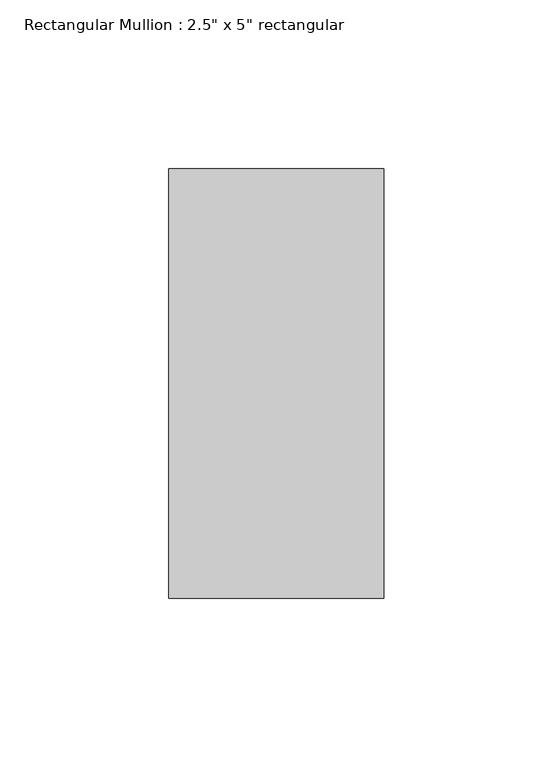
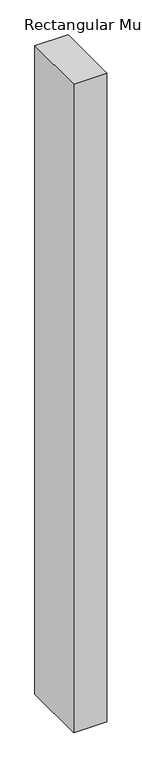
"""IFC4 building model written with IfcOpenShell, lengths in millimetres: member geometry."""

from ifc_helpers import new_model, si_unit, frame, origin, place, context, project, spatial, polyline, outline, extrude, source, transform, mapped, element, save


def member_13061b82(model_context):
    return source(origin(), model_context, "Body", "SweptSolid", [
        extrude(outline(polyline([(0.0, 63.5), (0.0, -63.5), (-63.5, -63.5), (-63.5, 63.5), (0.0, 63.5)])), frame((0.0, 0.0, -1301.7500001), z_axis=(0.0, 0.0, 1.0), x_axis=(1.0, 0.0, 0.0)), (0.0, 0.0, 1.0), 1301.7500001),
    ])


if __name__ == "__main__":
    model = new_model("IFC4")
    model_context = context("Model", 3, world=origin())
    ifc_project = project(units=[si_unit("LENGTHUNIT", "METRE", prefix="MILLI")], contexts=[model_context])
    site = spatial("IfcSite", under=ifc_project)
    building = spatial("IfcBuilding", under=site)
    placement = place(None, origin())
    member_shape = member_13061b82(model_context)
    element("IfcMember", 1, ObjectType="Rectangular Mullion : 2.5\" x 5\" rectangular", at=placement, inside=building, context=model_context, shape_type="MappedRepresentation", body=[
        mapped(member_shape, transform((0.0, 0.0, 0.0), x_axis=(1.0, 0.0, 0.0), y_axis=(0.0, 1.0, 0.0), z_axis=(0.0, 0.0, 1.0))),
    ])
    save(model, "model.ifc")

# Revit data of these elements
# Type "Rectangular Mullion : 2.5\" x 5\" rectangular"
#   built-in parameter 1007304 = 0.416667 (stored number, unit not read)
#   built-in parameter 1007301 = 0.104167 (stored number, unit not read)
#   built-in parameter 1007300 = 0.104167 (stored number, unit not read)
# Element 1 (IfcMember, "Rectangular Mullion : 2.5\" x 5\" rectangular")
#   Materials on its faces: "Aluminum"
# Materials
#   "Aluminum": class "Metal", colour RGB 247 247 247, transparency 0, Description = "Aluminum 6061", Cost = 0
